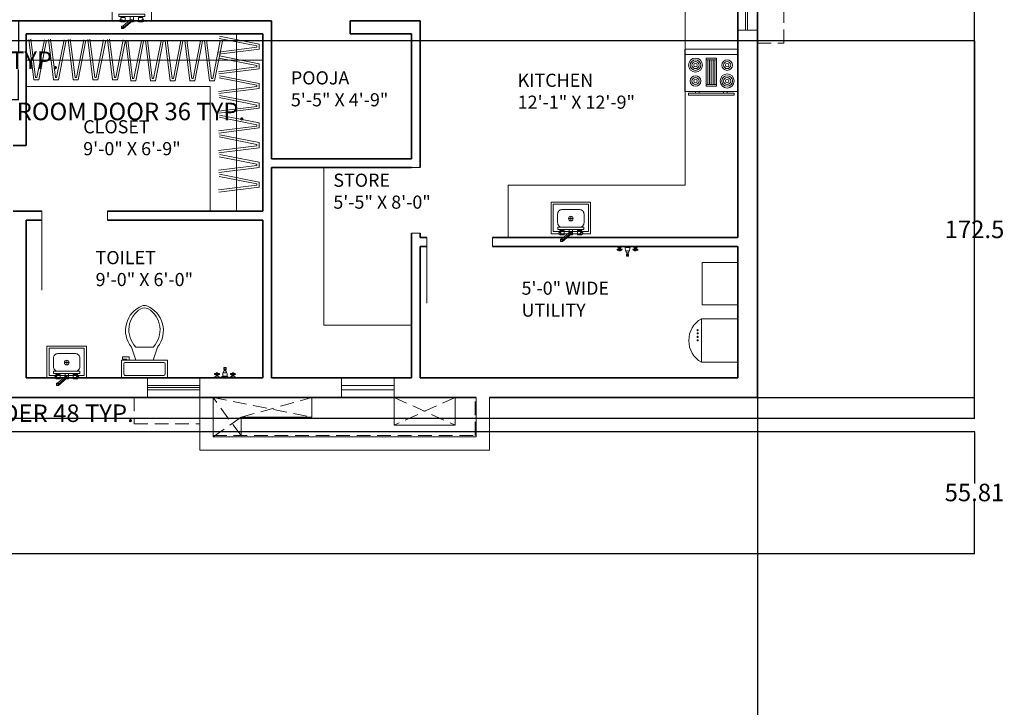
# Model space of a CAD drawing. Units: inches. Extents: x 3343 to 4790, y 1140 to 2641.
# Tile 8 of 10: x 4337 to 4787, y 1710 to 2024. Entities that reach past the tile are written whole.
import ezdxf

# ---------------------------------------------------------------- set-up
doc = ezdxf.new("R2010")
doc.units = ezdxf.units.IN
doc.header["$LTSCALE"] = 5
doc.header["$MEASUREMENT"] = 0
doc.linetypes.add('HIDDEN', pattern=[0.375, 0.25, -0.125])
for name, color, linetype, lineweight in [('A-ANNO-DIMS', 2, 'Continuous', 18), ('A-AREA-IDEN', 7, 'Continuous', 18), ('A-DOOR', 3, 'Continuous', 18), ('A-EQPM', 9, 'Continuous', 18), ('A-FLOR-CASE', 9, 'Continuous', 18), ('A-FLOR-FIXT', 9, 'Continuous', 18), ('A-FLOR-HIDN', 8, 'HIDDEN', 13), ('A-FLOR-SHFT', 8, 'Continuous', 18), ('A-GLAZ', 4, 'Continuous', 18), ('A-WALL', 7, 'Continuous', 35)]:
    doc.layers.add(name, color=color, linetype=linetype, lineweight=lineweight)
doc.styles.get("Standard").update_dxf_attribs({"font": 'arial.ttf'})
doc.dimstyles.get("Standard").update_dxf_attribs({"dimtxt": 8, "dimasz": 0.18, "dimexe": 0.18, "dimexo": 0.0625, "dimgap": 0.09, "dimtad": 0, "dimtih": 1, "dimtoh": 1, "dimdec": 1, "dimzin": 0, "dimdsep": 46, "dimlunit": 3, "dimtxsty": 'Standard', "dimcen": 0.09, "dimadec": 0, "dimazin": 0, "dimtfac": 1, "dimtdec": 1, "dimtofl": 0, "dimtmove": 0, "dimatfit": 3, "dimfxl": 1, "dimtolj": 1, "dimtzin": 0, "dimarcsym": 0})

# ---------------------------------------------------------------- blocks, each defined once
blk = doc.blocks.new('Toilet - top')
for p, q in [((9.5, -6), (9.5, -2)), ((-10, -8.5), (-8, -8.5)), ((-10, -9.5), (-10, -8.5)), ((-8, -8.5), (-8, -8)), ((-7, -8), (-7, -9.5)), ((-4, -8), (-6, -14)), ((4, -8), (6, -14)), ((-7, -9.5), (-10, -9.5)), ((4, -14), (-4, -14))]:
    blk.add_line(p, q)
blk.add_lwpolyline([(10.5, -8), (10.5, 0), (-10.5, 0), (-10.5, -8)], close=True)
for points in [[(-9.5, -2), (-9.5, -6)], [(8.5, -1), (-8.5, -1)], [(-8.5, -7), (8.5, -7)]]:
    blk.add_lwpolyline(points)
for centre, radius, start, end in [((-8.62, -1.88), 0.884, 81.8699, 188.1301), ((8.62, -1.88), 0.884, 351.8699, 98.1301), ((-8.62, -6.12), 0.884, 171.8699, 278.1301), ((8.62, -6.12), 0.884, 261.8699, 8.1301), ((3.52, -21.58), 12.17, 141.4691, 247.9714), ((4.2, -21.82), 11.33, 136.3677, 238.9468), ((-3.52, -21.58), 12.17, 292.0284, 38.5307), ((-4.2, -21.82), 11.33, 301.053, 43.6321), ((0, -27.88), 4, 245.7318, 294.2682), ((0, -29), 4, 254.8605, 285.1395)]:
    blk.add_arc(centre, radius, start, end)
blk = doc.blocks.new('Faucet - Bathroom front')
for p, q in [((-5, 0), (-2.25, 0)), ((-4.5087, 0.25), (-2.7408, 0.25)), ((-4, 1.625), (-4.25, 1.625)), ((-4, 1.375), (-4.25, 1.375)), ((-3.1442, 0.75), (-4.0979, 0.75)), ((-3.25, 1.625), (-3, 1.625)), ((-3.25, 1.375), (-3, 1.375)), ((-1.5, 0), (1.5, 0)), ((-1, 0.5), (1, 0.5)), ((-0.5, 4.25), (0.5, 4.25)), ((0.5, 3.75), (-0.5, 3.75)), ((-0.5, 3), (0.5, 3)), ((0.5, 2), (-0.5, 2)), ((-0.25, 3), (-0.25, 3.5)), ((0.25, 3.5), (0.25, 3)), ((2.25, 0), (5, 0)), ((2.7413, 0.25), (4.5092, 0.25)), ((3.25, 1.625), (3, 1.625)), ((3.25, 1.375), (3, 1.375)), ((4.1058, 0.75), (3.1521, 0.75)), ((4, 1.625), (4.25, 1.625)), ((4, 1.375), (4.25, 1.375))]:
    blk.add_line(p, q)
for points in [[(-0.25, 4.5), (0.25, 4.5)], [(-0.5, 3.75), (-0.5, 4.25)], [(0.25, 3.5), (-0.25, 3.5)], [(0.5, 4.25), (0.5, 3.75)]]:
    blk.add_lwpolyline(points)
for points in [[(-4, 1), (-4, 2), (-3.25, 2), (-3.25, 1)], [(3.25, 1), (3.25, 2), (4, 2), (4, 1)]]:
    blk.add_lwpolyline(points, close=True)
for centre in [(-4.5, 1.5), (-3.625, 1.5), (-2.75, 1.5), (2.75, 1.5), (3.625, 1.5), (4.5, 1.5)]:
    blk.add_circle(centre, 0.2795)
for centre, radius, start, end in [((-0.2575, 4.2575), 0.2426, 88.22243, 181.7776), ((0.2575, 4.2575), 0.2426, 358.2224, 91.77757), ((-5.375, 1.375), 1.4252, 285.2551, 344.7449), ((-1.875, 1.375), 1.4252, 195.2551, 254.7449), ((-0.7962, -0.2038), 0.7327, 106.1502, 163.8498), ((3, 1), 4.0311, 150.2551, 187.125), ((0.6413, 2.5), 1.246, 156.3417, 203.6583), ((-0.2575, 3.7425), 0.2426, 178.2224, 271.7776), ((0.2575, 3.7425), 0.2426, 268.2224, 1.777565), ((-3, 1), 4.0311, 352.875, 29.74488), ((-0.6413, 2.5), 1.246, 336.3417, 23.65835), ((0.7962, -0.2038), 0.7327, 16.1502, 73.84979), ((1.875, 1.375), 1.4252, 285.2551, 344.7449), ((5.375, 1.375), 1.4252, 195.2551, 254.7449)]:
    blk.add_arc(centre, radius, start, end)
blk = doc.blocks.new('Faucet - kit sink front')
for p, q in [((-0.25, 3), (3.75, 6.5)), ((3.75, 6), (-0.25, 2.5)), ((4.1921, 5.5041), (0.75, 2.5)), ((3.75, 6), (3.75, 6.5)), ((3.75, 6.5), (4.75, 6.5)), ((3.75, 5.5), (3.75, 6)), ((4.75, 6), (3.75, 6)), ((4.75, 5.5), (3.75, 5.5)), ((4.75, 6.5), (4.75, 6)), ((4.75, 6), (4.75, 5.5)), ((-4.5, 1), (-4.5, 1.5)), ((-3.5, 1.5), (-3.5, 1)), ((-0.75, 3.5), (0.3192, 3.5)), ((-0.75, 1), (-0.75, 3.5)), ((-0.25, 2.5), (-0.25, 3)), ((0.75, 2.5), (-0.25, 2.5)), ((0.75, 2.5), (0.75, 1)), ((3.5, 1.5), (3.5, 1)), ((4.5, 1), (4.5, 1.5))]:
    blk.add_line(p, q)
for points in [[(-6, 0), (-6, 1), (6, 1), (6, 0)], [(-5.5, 2.5), (-5.5, 3.25), (-4.5, 3.25), (-4.5, 2.5)], [(5.5, 2.5), (5.5, 3.25), (4.5, 3.25), (4.5, 2.5)]]:
    blk.add_lwpolyline(points, close=True)
for points in [[(-5, 3.2513), (-5, 3.5), (-3, 3.5), (-3, 1.5), (-5, 1.5), (-5, 2.5)], [(5, 3.2513), (5, 3.5), (3, 3.5), (3, 1.5), (5, 1.5), (5, 2.5)]]:
    blk.add_lwpolyline(points)
blk = doc.blocks.new('Range-Oven - 30 in top')
for p, q in [((0, -3), (30, -3)), ((12, -6), (18, -6)), ((13, -20), (13, -6)), ((14, -6), (14, -20)), ((15, -20), (15, -6)), ((16, -6), (16, -20)), ((17, -20), (17, -6)), ((18, -20), (12, -20)), ((6, -24), (6, -25)), ((8, -25), (8, -24)), ((22, -25), (22, -24)), ((24, -24), (24, -25))]:
    blk.add_line(p, q)
for points in [[(0, -24), (0, 0), (30, 0), (30, -24)], [(12, -21), (12, -5), (18, -5), (18, -21)], [(2, -26), (2, -25), (28, -25), (28, -26)]]:
    blk.add_lwpolyline(points, close=True)
for centre, radius in [((6, -9), 4), ((6, -9), 3), ((6, -9), 2), ((6, -9), 1), ((24, -9), 3), ((24, -9), 2), ((24, -9), 1), ((6, -18), 3), ((6, -18), 2), ((24, -18), 4), ((24, -18), 3), ((24, -18), 2), ((6, -18), 1), ((24, -18), 1)]:
    blk.add_circle(centre, radius)
blk = doc.blocks.new('UTILITY-APPLIANCE')
blk.add_lwpolyline([(22.35, 19.84), (5.78, 19.84), (5.78, 0), (22.35, 0)], close=True)
for centre in [(4.05, 14.66), (4.05, 13.23), (4.05, 11.58), (4.05, 10.02)]:
    blk.add_circle(centre, 0.275)
blk.add_arc((11.41, 9.92), 11.41, 119.598, 240.402)
blk = doc.blocks.new('WINDOW-48IN-SLIDING-JAMB9')
for p, q in [((0, 9), (0, 0)), ((48, 9), (48, 0)), ((0, 5.5), (24, 5.5)), ((0, 4.5), (48, 4.5)), ((24, 5.5), (24, 3.5)), ((24, 3.5), (48, 3.5))]:
    blk.add_line(p, q)
blk = doc.blocks.new('WINDOW-24IN-FIXED')
for p, q in [((0, 9), (0, 0)), ((24, 9), (24, 0)), ((0, 5.5), (24, 5.5)), ((0, 3.5), (24, 3.5))]:
    blk.add_line(p, q)
blk = doc.blocks.new('DOOR-30IN-4IN-JAMB')
for p, q in [((30, 30), (0, 30)), ((26, 30), (30, 30)), ((26, 0), (30, 0))]:
    blk.add_line(p, q)
blk = doc.blocks.new('WARDROBE-HANGER')
for points in [[(0.22, 7.19), (17.51, 3.78), (17.51, 3.18), (0, 0.99)], [(0.41, 8.17), (18.51, 4.61), (18.51, 2.3), (0.12, 0)]]:
    blk.add_lwpolyline(points)
blk = doc.blocks.new('*D47')
at = {"layer": 'A-ANNO-DIMS', "color": 0, "lineweight": -2, "ltscale": 5, "transparency": 16777216}
for p, q in [((4261.87, 1851.1), (4261.87, 1843.78)), ((4309.87, 1851.1), (4309.87, 1843.78)), ((4262.05, 1843.96), (4309.69, 1843.96)), ((4309.87, 1843.96), (4310.05, 1843.96))]:
    blk.add_line(p, q, dxfattribs=at)
at = {"layer": 'A-ANNO-DIMS', "color": 0, "ltscale": 5, "transparency": 16777216}
for points in [[(4262.05, 1843.99), (4262.05, 1843.93), (4261.87, 1843.96)], [(4309.69, 1843.99), (4309.69, 1843.93), (4309.87, 1843.96)]]:
    blk.add_solid(points, dxfattribs=at)
at = {"layer": 'Defpoints', "color": 0, "ltscale": 5, "transparency": 16777216}
for p in [(4261.87, 1851.16), (4309.87, 1851.16), (4309.87, 1843.96)]:
    blk.add_point(p, dxfattribs=at)
at = {"layer": 'A-ANNO-DIMS', "color": 0, "ltscale": 5, "transparency": 16777216, "insert": (4351.33, 1843.96), "char_height": 8, "attachment_point": 5}
blk.add_mtext('\\A1;SLIDER 48 TYP.', dxfattribs=at)
blk = doc.blocks.new('*D63')
at = {"layer": 'A-ANNO-DIMS', "color": 0, "lineweight": -2, "ltscale": 5, "transparency": 16777216}
for p, q in [((4295.13, 1987.1), (4295.13, 1981.58)), ((4331.13, 1987.1), (4331.13, 1981.58)), ((4295.31, 1981.76), (4330.95, 1981.76)), ((4331.13, 1981.76), (4331.31, 1981.76))]:
    blk.add_line(p, q, dxfattribs=at)
at = {"layer": 'A-ANNO-DIMS', "color": 0, "ltscale": 5, "transparency": 16777216}
for points in [[(4295.31, 1981.79), (4295.31, 1981.73), (4295.13, 1981.76)], [(4330.95, 1981.79), (4330.95, 1981.73), (4331.13, 1981.76)]]:
    blk.add_solid(points, dxfattribs=at)
at = {"layer": 'Defpoints', "color": 0, "ltscale": 5, "transparency": 16777216}
for p in [(4295.13, 1987.16), (4331.13, 1987.16), (4331.13, 1981.76)]:
    blk.add_point(p, dxfattribs=at)
at = {"layer": 'A-ANNO-DIMS', "color": 0, "ltscale": 5, "transparency": 16777216, "insert": (4387.92, 1981.76), "char_height": 8, "attachment_point": 5}
blk.add_mtext('\\A1;ROOM DOOR 36 TYP.', dxfattribs=at)
blk = doc.blocks.new('*D64')
at = {"layer": 'A-ANNO-DIMS', "color": 0, "lineweight": -2, "ltscale": 5, "transparency": 16777216}
for p, q in [((4331.19, 2023.16), (4336.71, 2023.16)), ((4336.53, 2022.98), (4336.53, 2009.34)), ((4336.53, 1987.34), (4336.53, 2000.98)), ((4331.19, 1987.16), (4336.71, 1987.16))]:
    blk.add_line(p, q, dxfattribs=at)
at = {"layer": 'A-ANNO-DIMS', "color": 0, "ltscale": 5, "transparency": 16777216}
for points in [[(4336.5, 2022.98), (4336.56, 2022.98), (4336.53, 2023.16)], [(4336.5, 1987.34), (4336.56, 1987.34), (4336.53, 1987.16)]]:
    blk.add_solid(points, dxfattribs=at)
at = {"layer": 'Defpoints', "color": 0, "ltscale": 5, "transparency": 16777216}
for p in [(4331.13, 2023.16), (4336.53, 2023.16), (4331.13, 1987.16)]:
    blk.add_point(p, dxfattribs=at)
at = {"layer": 'A-ANNO-DIMS', "color": 0, "ltscale": 5, "transparency": 16777216, "insert": (4336.53, 2005.16), "char_height": 8, "attachment_point": 5}
blk.add_mtext('\\A1;36 TYP.', dxfattribs=at)
blk = doc.blocks.new('*D86')
at = {"layer": 'A-ANNO-DIMS', "color": 0, "lineweight": -2, "ltscale": 5, "transparency": 16777216}
for p, q in [((4121.13, 1851.1), (4121.13, 1144.78)), ((4674.13, 1851.1), (4674.13, 1144.78)), ((4121.31, 1144.96), (4388.7, 1144.96)), ((4673.95, 1144.96), (4406.56, 1144.96))]:
    blk.add_line(p, q, dxfattribs=at)
at = {"layer": 'A-ANNO-DIMS', "color": 0, "ltscale": 5, "transparency": 16777216}
for points in [[(4121.31, 1144.99), (4121.31, 1144.93), (4121.13, 1144.96)], [(4673.95, 1144.99), (4673.95, 1144.93), (4674.13, 1144.96)]]:
    blk.add_solid(points, dxfattribs=at)
at = {"layer": 'Defpoints', "color": 0, "ltscale": 5, "transparency": 16777216}
for p in [(4121.13, 1851.16), (4674.13, 1851.16), (4674.13, 1144.96)]:
    blk.add_point(p, dxfattribs=at)
at = {"layer": 'A-ANNO-DIMS', "color": 0, "ltscale": 5, "transparency": 16777216, "insert": (4397.63, 1144.96), "char_height": 8, "attachment_point": 5}
blk.add_mtext('\\A1;553', dxfattribs=at)
blk = doc.blocks.new('*D87')
at = {"layer": 'A-ANNO-DIMS', "color": 0, "lineweight": -2, "ltscale": 5, "transparency": 16777216}
for p, q in [((3977.19, 2566.16), (4773.46, 2566.16)), ((4773.28, 2565.98), (4773.28, 2294.34)), ((4773.28, 2014.34), (4773.28, 2285.99)), ((3977.19, 2014.16), (4773.46, 2014.16))]:
    blk.add_line(p, q, dxfattribs=at)
at = {"layer": 'A-ANNO-DIMS', "color": 0, "ltscale": 5, "transparency": 16777216}
for points in [[(4773.25, 2565.98), (4773.31, 2565.98), (4773.28, 2566.16)], [(4773.25, 2014.34), (4773.31, 2014.34), (4773.28, 2014.16)]]:
    blk.add_solid(points, dxfattribs=at)
at = {"layer": 'Defpoints', "color": 0, "ltscale": 5, "transparency": 16777216}
for p in [(3977.13, 2566.16), (3977.13, 2014.16), (4773.28, 2014.16)]:
    blk.add_point(p, dxfattribs=at)
at = {"layer": 'A-ANNO-DIMS', "color": 0, "ltscale": 5, "transparency": 16777216, "insert": (4773.28, 2290.16), "char_height": 8, "attachment_point": 5}
blk.add_mtext('\\A1;552', dxfattribs=at)
blk = doc.blocks.new('*D88')
at = {"layer": 'A-ANNO-DIMS', "color": 0, "lineweight": -2, "ltscale": 5, "transparency": 16777216}
for p, q in [((4674.19, 2441.16), (4773.46, 2441.16)), ((4773.28, 2440.98), (4773.28, 2150.34)), ((4773.28, 1851.34), (4773.28, 2141.99)), ((4674.19, 1851.16), (4773.46, 1851.16))]:
    blk.add_line(p, q, dxfattribs=at)
at = {"layer": 'A-ANNO-DIMS', "color": 0, "ltscale": 5, "transparency": 16777216}
for points in [[(4773.25, 2440.98), (4773.31, 2440.98), (4773.28, 2441.16)], [(4773.25, 1851.34), (4773.31, 1851.34), (4773.28, 1851.16)]]:
    blk.add_solid(points, dxfattribs=at)
at = {"layer": 'Defpoints', "color": 0, "ltscale": 5, "transparency": 16777216}
for p in [(4674.13, 2441.16), (4773.28, 2441.16), (4674.13, 1851.16)]:
    blk.add_point(p, dxfattribs=at)
at = {"layer": 'A-ANNO-DIMS', "color": 0, "ltscale": 5, "transparency": 16777216, "insert": (4773.28, 2146.16), "char_height": 8, "attachment_point": 5}
blk.add_mtext('\\A1;590', dxfattribs=at)
blk = doc.blocks.new('*D95')
at = {"layer": 'A-ANNO-DIMS', "color": 0, "lineweight": -2, "ltscale": 5, "transparency": 16777216}
for p, q in [((3637.31, 2014.16), (4773.46, 2014.16)), ((4773.28, 2013.98), (4773.28, 1932.09)), ((4773.28, 1841.85), (4773.28, 1923.74)), ((3610.31, 1841.67), (4773.46, 1841.67))]:
    blk.add_line(p, q, dxfattribs=at)
at = {"layer": 'A-ANNO-DIMS', "color": 0, "ltscale": 5, "transparency": 16777216}
for points in [[(4773.25, 2013.98), (4773.31, 2013.98), (4773.28, 2014.16)], [(4773.25, 1841.85), (4773.31, 1841.85), (4773.28, 1841.67)]]:
    blk.add_solid(points, dxfattribs=at)
at = {"layer": 'Defpoints', "color": 0, "ltscale": 5, "transparency": 16777216}
for p in [(3637.25, 2014.16), (3610.25, 1841.67), (4773.28, 1841.67)]:
    blk.add_point(p, dxfattribs=at)
at = {"layer": 'A-ANNO-DIMS', "color": 0, "ltscale": 5, "transparency": 16777216, "insert": (4773.28, 1927.92), "char_height": 8, "attachment_point": 5}
blk.add_mtext('\\A1;172.5', dxfattribs=at)
blk = doc.blocks.new('*D98')
at = {"layer": 'A-ANNO-DIMS', "color": 0, "lineweight": -2, "ltscale": 5, "transparency": 16777216}
for p, q in [((3811.31, 1835.67), (4773.46, 1835.67)), ((4773.28, 1835.49), (4773.28, 1811.94)), ((4773.28, 1780.04), (4773.28, 1803.59)), ((3811.31, 1779.86), (4773.46, 1779.86))]:
    blk.add_line(p, q, dxfattribs=at)
at = {"layer": 'A-ANNO-DIMS', "color": 0, "ltscale": 5, "transparency": 16777216}
for points in [[(4773.25, 1835.49), (4773.31, 1835.49), (4773.28, 1835.67)], [(4773.25, 1780.04), (4773.31, 1780.04), (4773.28, 1779.86)]]:
    blk.add_solid(points, dxfattribs=at)
at = {"layer": 'Defpoints', "color": 0, "ltscale": 5, "transparency": 16777216}
for p in [(3811.25, 1835.67), (3811.25, 1779.86), (4773.28, 1779.86)]:
    blk.add_point(p, dxfattribs=at)
at = {"layer": 'A-ANNO-DIMS', "color": 0, "ltscale": 5, "transparency": 16777216, "insert": (4773.28, 1807.76), "char_height": 8, "attachment_point": 5}
blk.add_mtext('\\A1;55.81', dxfattribs=at)

msp = doc.modelspace()

# ---------------------------------------------------------------- linework, layer by layer
at = {"layer": 'A-DOOR'}
for p, q in [((4347.175, 1936.161), (4347.175, 1932.161)), ((4347.175, 1936.161), (4347.175, 1900.161)), ((4377.175, 1936.161), (4377.175, 1932.161))]:
    msp.add_line(p, q, dxfattribs=at)
at = {"layer": 'A-EQPM'}
msp.add_lwpolyline([(4665.13, 1912.73), (4648.908, 1912.73), (4648.908, 1893.506), (4665.13, 1893.506)], close=True, dxfattribs=at)
at = {"layer": 'A-FLOR-CASE'}
for p, q in [((4641.13, 2077.161), (4641.13, 1948.161)), ((4340.13, 2017.161), (4340.13, 2005.161)), ((4436.13, 1936.161), (4436.13, 2017.161)), ((4436.13, 2017.161), (4436.13, 1936.161)), ((4340.13, 2005.161), (4448.13, 2005.161)), ((4340.13, 1993.161), (4424.13, 1993.161)), ((4424.13, 1993.161), (4424.13, 1936.161)), ((4476.13, 1956.161), (4476.13, 1884.161)), ((4560.328, 1948.161), (4641.13, 1948.161)), ((4560.328, 1948.161), (4560.328, 1924.161)), ((4448.13, 1936.161), (4436.13, 1936.161)), ((4476.13, 1884.161), (4516.13, 1884.161))]:
    msp.add_line(p, q, dxfattribs=at)
at = {"layer": 'A-FLOR-FIXT'}
for p, q in [((4589.946, 1932.827), (4587.827, 1932.827)), ((4588.886, 1931.767), (4588.886, 1933.886)), ((4359.68, 1867.073), (4357.561, 1867.073)), ((4358.62, 1866.013), (4358.62, 1868.133))]:
    msp.add_line(p, q, dxfattribs=at)
for points in [[(4379.334, 2023.161), (4379.334, 2037.598), (4397.396, 2037.598), (4397.396, 2023.161)], [(4579.855, 1925.915), (4579.855, 1940.351), (4597.918, 1940.351), (4597.918, 1925.915)], [(4580.855, 1939.351), (4596.918, 1939.351), (4596.918, 1926.915), (4580.855, 1926.915)], [(4349.589, 1860.161), (4349.589, 1874.598), (4367.652, 1874.598), (4367.652, 1860.161)], [(4350.589, 1873.598), (4366.652, 1873.598), (4366.652, 1861.161), (4350.589, 1861.161)]]:
    msp.add_lwpolyline(points, close=True, dxfattribs=at)
for points in [[(4594.918, 1930.915), (4594.918, 1934.915, 0.4142136), (4592.918, 1936.915), (4584.855, 1936.915, 0.4142136), (4582.855, 1934.915), (4582.855, 1930.915, 0.4142136), (4584.855, 1928.915), (4592.918, 1928.915, 0.4142136)], [(4364.652, 1865.161), (4364.652, 1869.161, 0.4142136), (4362.652, 1871.161), (4354.589, 1871.161, 0.4142136), (4352.589, 1869.161), (4352.589, 1865.161, 0.4142136), (4354.589, 1863.161), (4362.652, 1863.161, 0.4142136)]]:
    msp.add_lwpolyline(points, format="xyb", close=True, dxfattribs=at)
for centre in [(4588.886, 1932.827), (4358.62, 1867.073)]:
    msp.add_circle(centre, 1.06, dxfattribs=at)
at = {"layer": 'A-FLOR-HIDN', "ltscale": 5}
for p, q in [((4686.13, 2012.896), (4686.13, 2066.896)), ((4674.13, 2018.896), (4674.13, 2012.896)), ((4674.13, 2012.896), (4686.13, 2012.896)), ((4395.464, 1851.161), (4389.464, 1851.161)), ((4389.464, 1851.161), (4389.464, 1839.161)), ((4438.244, 1833.711), (4425.464, 1851.161)), ((4425.464, 1851.161), (4470.618, 1842.098)), ((4438.244, 1842.098), (4470.618, 1851.161)), ((4508.13, 1851.161), (4536.031, 1838.526)), ((4536.031, 1851.161), (4508.13, 1838.526)), ((4545.192, 1833.711), (4545.192, 1851.161)), ((4425.464, 1833.161), (4438.244, 1842.098)), ((4389.464, 1839.161), (4419.464, 1839.161)), ((4425.464, 1833.711), (4545.192, 1833.711))]:
    msp.add_line(p, q, dxfattribs=at)
at = {"layer": 'A-FLOR-SHFT', "ltscale": 5}
for p, q in [((4419.464, 1851.161), (4419.464, 1827.161)), ((4425.464, 1851.161), (4425.464, 1833.161)), ((4470.618, 1851.161), (4470.618, 1842.098)), ((4470.618, 1842.098), (4438.244, 1842.098)), ((4438.244, 1842.098), (4438.244, 1833.711))]:
    msp.add_line(p, q, dxfattribs=at)
at = {"layer": 'A-FLOR-SHFT'}
for p, q in [((4545.72, 1833.161), (4545.72, 1851.161)), ((4551.72, 1827.161), (4551.72, 1851.161)), ((4425.464, 1833.161), (4545.72, 1833.161)), ((4419.464, 1827.161), (4551.72, 1827.161))]:
    msp.add_line(p, q, dxfattribs=at)
msp.add_lwpolyline([(4508.13, 1851.161), (4536.031, 1851.161), (4536.031, 1838.526), (4508.13, 1838.526)], close=True, dxfattribs=at)
at = {"layer": 'A-GLAZ'}
for p, q in [((4395.464, 1860.161), (4395.464, 1851.161)), ((4419.464, 1860.161), (4419.464, 1851.161)), ((4395.464, 1856.661), (4419.464, 1856.661)), ((4395.464, 1855.661), (4419.464, 1855.661)), ((4395.464, 1854.661), (4419.464, 1854.661))]:
    msp.add_line(p, q, dxfattribs=at)
at = {"layer": 'A-WALL'}
for p, q in [((4674.13, 2441.161), (4674.13, 1851.161)), ((4665.13, 2077.161), (4665.13, 1924.161)), ((4331.13, 2023.161), (4452.13, 2023.161)), ((4452.13, 2017.161), (4452.13, 2023.161)), ((4488.13, 2017.161), (4488.13, 2023.161)), ((4488.13, 2023.161), (4520.13, 2023.161)), ((4520.13, 2023.161), (4520.13, 2017.161)), ((4520.13, 2023.161), (4520.13, 2017.161)), ((4520.13, 2023.161), (4520.13, 1956.161)), ((4340.13, 2017.161), (4340.13, 1966.161)), ((4340.13, 2017.161), (4448.13, 2017.161)), ((4448.13, 2017.161), (4448.13, 1936.161)), ((4452.13, 2017.161), (4452.13, 1960.161)), ((4488.13, 2017.161), (4516.13, 2017.161)), ((4516.13, 2017.161), (4516.13, 1960.161)), ((4340.13, 1966.161), (4334.13, 1966.161)), ((4452.13, 1960.161), (4516.13, 1960.161)), ((4452.13, 1956.161), (4516.13, 1956.161)), ((4452.13, 1956.161), (4452.13, 1860.161)), ((4340.13, 1936.161), (4334.13, 1936.161)), ((4340.13, 1936.161), (4347.175, 1936.161)), ((4377.175, 1936.161), (4448.13, 1936.161)), ((4340.13, 1932.161), (4347.175, 1932.161)), ((4340.13, 1932.161), (4340.13, 1860.161)), ((4377.175, 1932.161), (4448.13, 1932.161)), ((4448.13, 1932.161), (4448.13, 1860.161)), ((4516.13, 1926.161), (4516.13, 1860.161)), ((4520.13, 1926.161), (4520.13, 1924.161)), ((4520.13, 1924.161), (4523.13, 1924.161)), ((4553.13, 1924.161), (4665.13, 1924.161)), ((4520.13, 1920.161), (4523.13, 1920.161)), ((4520.13, 1920.161), (4520.13, 1860.161)), ((4553.13, 1920.161), (4665.13, 1920.161)), ((4665.13, 1920.161), (4665.13, 1860.161)), ((4340.13, 1860.161), (4448.13, 1860.161)), ((4452.13, 1860.161), (4516.13, 1860.161)), ((4520.13, 1860.161), (4665.13, 1860.161)), ((4309.873, 1851.161), (4545.72, 1851.161)), ((4551.72, 1851.161), (4674.13, 1851.161))]:
    msp.add_line(p, q, dxfattribs=at)

# ---------------------------------------------------------------- block references
at = {"layer": 'A-DOOR'}
msp.add_blockref('DOOR-30IN-4IN-JAMB', (4490.13, 1926.161), dxfattribs=at)
at = {"layer": 'A-DOOR', "rotation": 89.99999999999737}
msp.add_blockref('DOOR-30IN-4IN-JAMB', (4553.13, 1894.161), dxfattribs=at)
at = {"layer": 'A-EQPM', "xscale": 0.8038317938248679, "yscale": 0.8038317938248679, "zscale": 0.8038317938248679}
msp.add_blockref('Range-Oven - 30 in top', (4641.02, 2010.152), dxfattribs=at)
at = {"layer": 'A-EQPM'}
msp.add_blockref('UTILITY-APPLIANCE', (4642.775, 1867.226), dxfattribs=at)
at = {"layer": 'A-FLOR-CASE'}
for p in [(4427.963, 2007.918), (4427.963, 1998.918), (4427.963, 1989.918), (4427.963, 1980.918), (4427.963, 1971.918), (4427.963, 1962.918), (4427.963, 1953.918), (4427.963, 1944.918)]:
    msp.add_blockref('WARDROBE-HANGER', p, dxfattribs=at)
for p, rotation in [((4341.235, 2014.716), 270.0000000000045), ((4350.235, 2014.716), 270.0000000000094), ((4359.235, 2014.716), 270.0000000000045), ((4368.235, 2014.716), 269.9999999999996), ((4377.235, 2014.716), 270.0000000000045), ((4385.54, 2014.273), 270.0000000000056), ((4394.54, 2014.273), 270.0000000000056), ((4403.54, 2014.273), 270.0000000000056), ((4412.54, 2014.273), 270.0000000000104), ((4421.54, 2014.273), 270.0000000000007)]:
    msp.add_blockref('WARDROBE-HANGER', p, dxfattribs=dict(at, rotation=rotation))
at = {"layer": 'A-FLOR-FIXT', "rotation": 180}
for name, p in [('Faucet - kit sink front', (4388.365, 2026.161)), ('Faucet - kit sink front', (4588.886, 1928.915)), ('Faucet - Bathroom front', (4614.795, 1920.161)), ('Faucet - kit sink front', (4358.62, 1863.161))]:
    msp.add_blockref(name, p, dxfattribs=at)
at = {"layer": 'A-FLOR-FIXT', "xscale": -1, "rotation": 180}
msp.add_blockref('Toilet - top', (4394.13, 1860.161), dxfattribs=at)
at = {"layer": 'A-FLOR-FIXT'}
msp.add_blockref('Faucet - Bathroom front', (4430.891, 1860.365), dxfattribs=at)
at = {"layer": 'A-GLAZ', "rotation": 90.00000000000138}
msp.add_blockref('WINDOW-48IN-SLIDING-JAMB9', (4674.13, 2018.896), dxfattribs=at)
at = {"layer": 'A-GLAZ'}
msp.add_blockref('WINDOW-24IN-FIXED', (4484.13, 1851.161), dxfattribs=at)

# ---------------------------------------------------------------- texts
at = {"layer": 'A-AREA-IDEN', "ltscale": 5, "char_height": 6, "attachment_point": 1}
for s, insert in [('POOJA\\P5\'-5" X 4\'-9"', (4461.019, 2000.095)), ('KITCHEN\\P12\'-1" X 12\'-9"', (4564.608, 1998.997)), ('CLOSET\\P9\'-0" X 6\'-9"', (4366.155, 1977.769)), ('STORE\\P5\'-5" X 8\'-0"', (4480.404, 1953.358)), ('TOILET\\P9\'-0" X 6\'-0"', (4371.806, 1918.011)), ('5\'-0" WIDE\\PUTILITY', (4566.384, 1904.061))]:
    msp.add_mtext_dynamic_manual_height_columns(s, width=189.69543, gutter_width=1, heights=[0], dxfattribs=dict(at, insert=insert))

# ---------------------------------------------------------------- dimensions: what is measured, and where the dimension line sits
at = {"layer": 'A-ANNO-DIMS', "ltscale": 5}
for base, p1, p2, override, picture, middle in [((4773.28, 2014.161), (3977.13, 2566.161), (3977.13, 2014.161), {"dimdec": 0, "dimlfac": 1, "dimrnd": 0, "dimzin": 0, "dimdsep": 46, "dimlunit": 2}, '*D87', (4773.28, 2290.161)), ((4773.28, 2441.161), (4674.13, 1851.161), (4674.13, 2441.161), {"dimdec": 0, "dimlfac": 1, "dimrnd": 0, "dimzin": 0, "dimdsep": 46, "dimlunit": 2}, '*D88', (4773.28, 2146.161)), ((4773.28, 1841.669), (3637.248, 2014.161), (3610.248, 1841.669), {"dimdec": 1, "dimlfac": 1, "dimrnd": 0, "dimzin": 0, "dimdsep": 46, "dimlunit": 2}, '*D95', (4773.28, 1927.915)), ((4773.28, 1779.857), (3811.248, 1835.669), (3811.248, 1779.857), {"dimdec": 2, "dimlfac": 1, "dimrnd": 0, "dimzin": 0, "dimdsep": 46, "dimlunit": 2}, '*D98', (4773.28, 1807.763))]:
    dim = msp.add_linear_dim(base=base, p1=p1, p2=p2, angle=90, dimstyle='Standard', override=override, dxfattribs=at)
    dim.commit()
    dim.dimension.update_dxf_attribs({"geometry": picture, "text_midpoint": middle})
dim = msp.add_linear_dim(base=(4336.53, 2023.161), p1=(4331.13, 1987.161), p2=(4331.13, 2023.161), angle=90, text='<> TYP.', dimstyle='Standard', override={"dimdec": 0, "dimlfac": 1, "dimrnd": 0, "dimzin": 0, "dimdsep": 46, "dimlunit": 2}, dxfattribs=at)
dim.commit()
dim.dimension.update_dxf_attribs({"geometry": '*D64', "text_midpoint": (4336.53, 2005.161)})
for base, p1, p2, text, picture, middle in [((4331.13, 1981.761), (4295.13, 1987.161), (4331.13, 1987.161), 'ROOM DOOR <> TYP.', '*D63', (4387.915, 1981.761)), ((4309.873, 1843.961), (4261.873, 1851.161), (4309.873, 1851.161), 'SLIDER <> TYP.', '*D47', (4351.333, 1843.961))]:
    dim = msp.add_linear_dim(base=base, p1=p1, p2=p2, text=text, dimstyle='Standard', override={"dimdec": 0, "dimlfac": 1, "dimrnd": 0, "dimzin": 0, "dimdsep": 46, "dimlunit": 2}, dxfattribs=at)
    dim.commit()
    dim.dimension.update_dxf_attribs({"geometry": picture, "text_midpoint": middle})
dim = msp.add_linear_dim(base=(4674.13, 1144.962), p1=(4121.13, 1851.161), p2=(4674.13, 1851.161), dimstyle='Standard', override={"dimdec": 0, "dimlfac": 1, "dimrnd": 0, "dimzin": 0, "dimdsep": 46, "dimlunit": 2}, dxfattribs=at)
dim.commit()
dim.dimension.update_dxf_attribs({"geometry": '*D86', "text_midpoint": (4397.63, 1144.962)})

doc.saveas('drawing.dxf')
